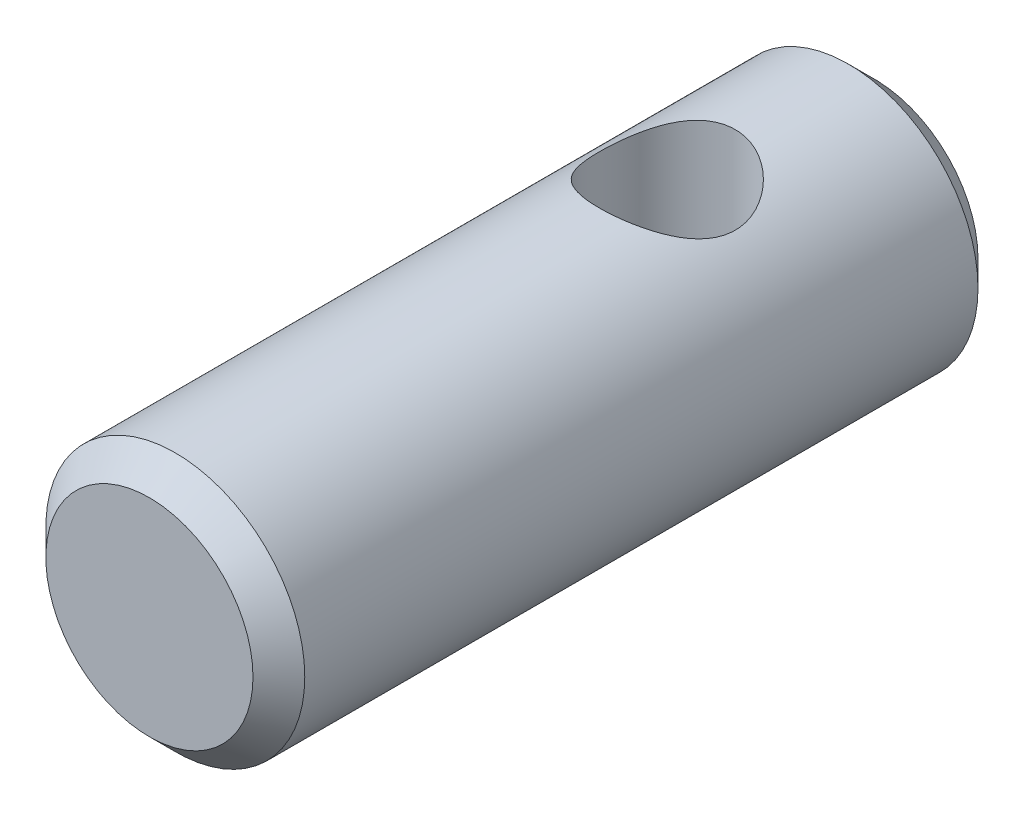
ISO-10303-21;
HEADER;
FILE_DESCRIPTION(('STEP AP214'),'2;1');
FILE_NAME('part.step','',(''),(''),'','','');
FILE_SCHEMA(('AUTOMOTIVE_DESIGN { 1 0 10303 214 1 1 1 1 }'));
ENDSEC;
DATA;
#1=APPLICATION_CONTEXT('core data for automotive mechanical design processes');
#2=APPLICATION_PROTOCOL_DEFINITION('international standard','automotive_design',2000,#1);
#3=PRODUCT_CONTEXT('',#1,'mechanical');
#4=PRODUCT('Part','Part','',(#3));
#5=PRODUCT_RELATED_PRODUCT_CATEGORY('part','',(#4));
#6=PRODUCT_DEFINITION_FORMATION('','',#4);
#7=PRODUCT_DEFINITION_CONTEXT('part definition',#1,'design');
#8=PRODUCT_DEFINITION('design','',#6,#7);
#9=PRODUCT_DEFINITION_SHAPE('','',#8);
#10=(LENGTH_UNIT() NAMED_UNIT(*) SI_UNIT(.MILLI.,.METRE.));
#11=(NAMED_UNIT(*) PLANE_ANGLE_UNIT() SI_UNIT($,.RADIAN.));
#12=(NAMED_UNIT(*) SI_UNIT($,.STERADIAN.) SOLID_ANGLE_UNIT());
#13=UNCERTAINTY_MEASURE_WITH_UNIT(LENGTH_MEASURE(1.E-05),#10,'distance_accuracy_value','');
#14=(GEOMETRIC_REPRESENTATION_CONTEXT(3) GLOBAL_UNCERTAINTY_ASSIGNED_CONTEXT((#13)) GLOBAL_UNIT_ASSIGNED_CONTEXT((#10,
#11,#12)) REPRESENTATION_CONTEXT('',''));
#15=CARTESIAN_POINT('',(0.,0.,0.));
#16=DIRECTION('',(0.,0.,1.));
#17=DIRECTION('',(1.,0.,0.));
#18=AXIS2_PLACEMENT_3D('',#15,#16,#17);
#19=CARTESIAN_POINT('',(0.,0.,56.));
#20=DIRECTION('',(0.,0.,-1.));
#21=DIRECTION('',(-1.,0.,0.));
#22=AXIS2_PLACEMENT_3D('',#19,#20,#21);
#23=CYLINDRICAL_SURFACE('',#22,10.);
#24=CARTESIAN_POINT('',(0.,0.,54.));
#25=DIRECTION('',(0.,0.,1.));
#26=DIRECTION('',(1.,0.,0.));
#27=AXIS2_PLACEMENT_3D('',#24,#25,#26);
#28=CIRCLE('',#27,10.);
#29=CARTESIAN_POINT('',(10.,0.,54.));
#30=VERTEX_POINT('',#29);
#31=EDGE_CURVE('E50',#30,#30,#28,.F.);
#32=ORIENTED_EDGE('',*,*,#31,.T.);
#33=EDGE_LOOP('',(#32));
#34=FACE_BOUND('',#33,.T.);
#35=CARTESIAN_POINT('',(0.,0.,1.99999999999999));
#36=DIRECTION('',(0.,0.,1.));
#37=DIRECTION('',(1.,0.,0.));
#38=AXIS2_PLACEMENT_3D('',#35,#36,#37);
#39=CIRCLE('',#38,10.);
#40=CARTESIAN_POINT('',(10.,0.,1.99999999999999));
#41=VERTEX_POINT('',#40);
#42=EDGE_CURVE('E51',#41,#41,#39,.T.);
#43=ORIENTED_EDGE('',*,*,#42,.T.);
#44=EDGE_LOOP('',(#43));
#45=FACE_BOUND('',#44,.T.);
#46=CARTESIAN_POINT('',(0.,-10.,21.25));
#47=CARTESIAN_POINT('',(0.137219280547153,-10.0000002272335,21.2500002845405));
#48=CARTESIAN_POINT('',(0.274435419117508,-9.9971695390607,21.244614606331));
#49=CARTESIAN_POINT('',(0.547846222323781,-9.98591963414679,21.2231383953593));
#50=CARTESIAN_POINT('',(0.684040493235206,-9.97749836499467,21.2070439311885));
#51=CARTESIAN_POINT('',(0.954484268200273,-9.95526954825004,21.1643222587016));
#52=CARTESIAN_POINT('',(1.08873124630636,-9.94145555844572,21.1376824522521));
#53=CARTESIAN_POINT('',(1.35420731073398,-9.90878502481806,21.0741759100838));
#54=CARTESIAN_POINT('',(1.48543513996533,-9.88992642039346,21.037304994978));
#55=CARTESIAN_POINT('',(1.74338589936232,-9.84772073139797,20.953926916141));
#56=CARTESIAN_POINT('',(1.87012634391849,-9.82439408650479,20.9074635617848));
#57=CARTESIAN_POINT('',(2.11899910335566,-9.77374047241918,20.8052537810732));
#58=CARTESIAN_POINT('',(2.24112965821982,-9.74641199440784,20.7495038522873));
#59=CARTESIAN_POINT('',(2.59949324496559,-9.65934198911403,20.5690867282639));
#60=CARTESIAN_POINT('',(2.82796520762876,-9.59447028649094,20.4311649077595));
#61=CARTESIAN_POINT('',(3.27372275797712,-9.45204211778156,20.1139922398255));
#62=CARTESIAN_POINT('',(3.48932750449225,-9.37393643487358,19.9326443666005));
#63=CARTESIAN_POINT('',(3.8886458044364,-9.21545596865336,19.5383334829643));
#64=CARTESIAN_POINT('',(4.07233236069242,-9.13507933066736,19.3253439890081));
#65=CARTESIAN_POINT('',(4.41885642960393,-8.97292923888063,18.8512480626824));
#66=CARTESIAN_POINT('',(4.57845425792897,-8.89165111021945,18.5875602559427));
#67=CARTESIAN_POINT('',(4.78231536149079,-8.78267726364413,18.1716075663925));
#68=CARTESIAN_POINT('',(4.84436102124095,-8.74850075709137,18.0295030388187));
#69=CARTESIAN_POINT('',(4.95595024092318,-8.68577293511993,17.7393030342969));
#70=CARTESIAN_POINT('',(5.00550154057647,-8.65721813970725,17.5912113324525));
#71=CARTESIAN_POINT('',(5.08878465482483,-8.60851077322863,17.2993729510763));
#72=CARTESIAN_POINT('',(5.12330119908315,-8.58794984553599,17.1559180994452));
#73=CARTESIAN_POINT('',(5.18020997914699,-8.55374369431526,16.8658774929062));
#74=CARTESIAN_POINT('',(5.20260898139194,-8.54009461148355,16.7192935329284));
#75=CARTESIAN_POINT('',(5.23492209789572,-8.52032581020631,16.4243606895251));
#76=CARTESIAN_POINT('',(5.24484570818525,-8.51420036499284,16.2760132353741));
#77=CARTESIAN_POINT('',(5.25205946869656,-8.50975281069956,15.9789018663673));
#78=CARTESIAN_POINT('',(5.24935106056602,-8.51142981115412,15.8301380009715));
#79=CARTESIAN_POINT('',(5.23257907023163,-8.5217479943958,15.5537912805343));
#80=CARTESIAN_POINT('',(5.22010486854874,-8.52941410986321,15.426071367475));
#81=CARTESIAN_POINT('',(5.18592245284569,-8.55024031855141,15.1722883834829));
#82=CARTESIAN_POINT('',(5.16421138189128,-8.56340211154436,15.0462258376151));
#83=CARTESIAN_POINT('',(5.11181617148469,-8.59478129237691,14.7966330629832));
#84=CARTESIAN_POINT('',(5.08113266753343,-8.61299832215873,14.6731026555353));
#85=CARTESIAN_POINT('',(5.01112590957965,-8.65391561205324,14.4292574721334));
#86=CARTESIAN_POINT('',(4.97179923690138,-8.67661764578174,14.3089439897666));
#87=CARTESIAN_POINT('',(4.83944266050791,-8.75158613496986,13.9484926319502));
#88=CARTESIAN_POINT('',(4.7331971950735,-8.80998221055456,13.7143322078009));
#89=CARTESIAN_POINT('',(4.48927913110239,-8.93673383412094,13.2661129763646));
#90=CARTESIAN_POINT('',(4.35159249631468,-9.00509382533885,13.0520632074793));
#91=CARTESIAN_POINT('',(4.02599923880666,-9.15575739072048,12.6180678022914));
#92=CARTESIAN_POINT('',(3.83374090515359,-9.23866411313319,12.4015852559708));
#93=CARTESIAN_POINT('',(3.41536670121867,-9.40135838816874,12.0023342528049));
#94=CARTESIAN_POINT('',(3.18923148995555,-9.48114412592955,11.8195851889832));
#95=CARTESIAN_POINT('',(2.821282740588,-9.59469562525509,11.5698133976322));
#96=CARTESIAN_POINT('',(2.68996216013096,-9.63242744398394,11.4888434006179));
#97=CARTESIAN_POINT('',(2.41986332749828,-9.70379978677848,11.3383880146168));
#98=CARTESIAN_POINT('',(2.28108827753964,-9.73744204764833,11.2688977457436));
#99=CARTESIAN_POINT('',(1.99703485726557,-9.79964224031448,11.1421678788624));
#100=CARTESIAN_POINT('',(1.85175947518982,-9.82820247889612,11.0849227202681));
#101=CARTESIAN_POINT('',(1.55574231468487,-9.87938315597843,10.9833638548017));
#102=CARTESIAN_POINT('',(1.40500124075675,-9.90200435691644,10.939048487957));
#103=CARTESIAN_POINT('',(1.11282934307188,-9.93888050639706,10.8672906984546));
#104=CARTESIAN_POINT('',(0.971749460230005,-9.95369724432438,10.8387051082509));
#105=CARTESIAN_POINT('',(0.687234152071724,-9.97737832564566,10.7931815930195));
#106=CARTESIAN_POINT('',(0.543798965935319,-9.98624326965873,10.7762424926943));
#107=CARTESIAN_POINT('',(0.255835151509784,-9.9977649691323,10.7542501032815));
#108=CARTESIAN_POINT('',(0.111307032752615,-10.0004244577754,10.7491915814063));
#109=CARTESIAN_POINT('',(-0.177649036404393,-9.99946551039621,10.7510180045486));
#110=CARTESIAN_POINT('',(-0.322076991762344,-9.99584741118279,10.7579023088026));
#111=CARTESIAN_POINT('',(-0.596977627902548,-9.98302883233932,10.7823894009097));
#112=CARTESIAN_POINT('',(-0.727564346720147,-9.97434520954031,10.7990002755381));
#113=CARTESIAN_POINT('',(-0.986752417901722,-9.95204728968371,10.8418917496917));
#114=CARTESIAN_POINT('',(-1.11535313429704,-9.93843144599325,10.8681753824162));
#115=CARTESIAN_POINT('',(-1.36965004237689,-9.90658705292847,10.9301208766084));
#116=CARTESIAN_POINT('',(-1.4953471268205,-9.88835994251531,10.9657798126174));
#117=CARTESIAN_POINT('',(-1.74314372577149,-9.84770291270563,11.0461184149203));
#118=CARTESIAN_POINT('',(-1.86524183923142,-9.82527138093231,11.0908015424625));
#119=CARTESIAN_POINT('',(-2.23123711650007,-9.75112230193064,11.240316825719));
#120=CARTESIAN_POINT('',(-2.46841439744369,-9.69338463506806,11.3590433850495));
#121=CARTESIAN_POINT('',(-2.92006961741366,-9.56704734835907,11.6290622439496));
#122=CARTESIAN_POINT('',(-3.13453840111886,-9.49844337518584,11.7803676042087));
#123=CARTESIAN_POINT('',(-3.55886678955075,-9.34827580923661,12.1295715799768));
#124=CARTESIAN_POINT('',(-3.76585720791017,-9.26610842953409,12.3307004883061));
#125=CARTESIAN_POINT('',(-4.14465083180736,-9.10299232838763,12.7646733438667));
#126=CARTESIAN_POINT('',(-4.31642352057216,-9.02204471969024,12.9975445078946));
#127=CARTESIAN_POINT('',(-4.54921678298438,-8.90577435633367,13.3749564890276));
#128=CARTESIAN_POINT('',(-4.6244388087147,-8.86683357688885,13.5098103007094));
#129=CARTESIAN_POINT('',(-4.76308083496289,-8.7931345699769,13.7865235798825));
#130=CARTESIAN_POINT('',(-4.82650617229413,-8.75837445370803,13.9283798425349));
#131=CARTESIAN_POINT('',(-4.94081379482617,-8.69440356931228,14.2181203619124));
#132=CARTESIAN_POINT('',(-4.99170730203359,-8.66518784171106,14.3659990863072));
#133=CARTESIAN_POINT('',(-5.08032094735002,-8.61353453429228,14.6668057821361));
#134=CARTESIAN_POINT('',(-5.11804336108919,-8.59109578367589,14.8197328763379));
#135=CARTESIAN_POINT('',(-5.17667803179201,-8.55587841408529,15.114123629598));
#136=CARTESIAN_POINT('',(-5.19887396728424,-8.54236940354325,15.2552448007445));
#137=CARTESIAN_POINT('',(-5.23170136755015,-8.52230458141236,15.5393099760195));
#138=CARTESIAN_POINT('',(-5.24233433352715,-8.51574786721987,15.6822537410848));
#139=CARTESIAN_POINT('',(-5.25185951233148,-8.50987680634923,15.9686108559526));
#140=CARTESIAN_POINT('',(-5.25075745481041,-8.51055892529399,16.1120239424167));
#141=CARTESIAN_POINT('',(-5.23684562254051,-8.51912638319485,16.398056141514));
#142=CARTESIAN_POINT('',(-5.22403653550511,-8.52701129903249,16.5406753002904));
#143=CARTESIAN_POINT('',(-5.18905861916022,-8.54833517431968,16.8075526419432));
#144=CARTESIAN_POINT('',(-5.16813575164992,-8.5610310262324,16.9320359741887));
#145=CARTESIAN_POINT('',(-5.11754218486671,-8.59136907943889,17.1786107034704));
#146=CARTESIAN_POINT('',(-5.0878688274224,-8.60901278368161,17.3007013616383));
#147=CARTESIAN_POINT('',(-4.98617367311396,-8.66858187281142,17.6622746890925));
#148=CARTESIAN_POINT('',(-4.90145556802352,-8.71715897973571,17.8972171923239));
#149=CARTESIAN_POINT('',(-4.69456138578904,-8.83039079036659,18.3650285592195));
#150=CARTESIAN_POINT('',(-4.57029454343953,-8.89589043768955,18.5967527275334));
#151=CARTESIAN_POINT('',(-4.28992761428728,-9.03443201618363,19.0376472698748));
#152=CARTESIAN_POINT('',(-4.13381040597987,-9.10747799349605,19.2468054204548));
#153=CARTESIAN_POINT('',(-3.76892931535455,-9.26498416164771,19.6668056172768));
#154=CARTESIAN_POINT('',(-3.55586671949328,-9.34962231131358,19.8738577757245));
#155=CARTESIAN_POINT('',(-3.09590888201791,-9.51181668814184,20.2504194945182));
#156=CARTESIAN_POINT('',(-2.84899294804858,-9.58936853521662,20.4199059262879));
#157=CARTESIAN_POINT('',(-2.45489845847901,-9.69497778028643,20.6432164783478));
#158=CARTESIAN_POINT('',(-2.31807696854077,-9.72867771558496,20.7130413299976));
#159=CARTESIAN_POINT('',(-2.03793218201021,-9.79118868583265,20.8407633736319));
#160=CARTESIAN_POINT('',(-1.89461212988962,-9.82000212708188,20.8986664393929));
#161=CARTESIAN_POINT('',(-1.60279401104823,-9.8718274054918,21.001745186262));
#162=CARTESIAN_POINT('',(-1.45430732159531,-9.8948511724765,21.0469470615697));
#163=CARTESIAN_POINT('',(-1.15317060054867,-9.9344468208744,21.1241423051091));
#164=CARTESIAN_POINT('',(-1.00052299145191,-9.95102237408543,21.1561431909917));
#165=CARTESIAN_POINT('',(-0.706948892559235,-9.9759631073553,21.2041056127254));
#166=CARTESIAN_POINT('',(-0.566275097942629,-9.98495530017708,21.2212954311786));
#167=CARTESIAN_POINT('',(-0.283733098336377,-9.99697368746327,21.2442425896913));
#168=CARTESIAN_POINT('',(-0.141864870006832,-9.99999976507347,21.2499997058263));
#169=CARTESIAN_POINT('',(0.,-10.,21.25));
#170=B_SPLINE_CURVE_WITH_KNOTS('',3,(#46,#47,#48,#49,#50,#51,#52,#53,#54,#55,#56,#57,#58,#59,
#60,#61,#62,#63,#64,#65,#66,#67,#68,#69,#70,#71,#72,#73,#74,#75,#76,#77,#78,#79,#80,#81,#82,#83,
#84,#85,#86,#87,#88,#89,#90,#91,#92,#93,#94,#95,#96,#97,#98,#99,#100,#101,#102,#103,#104,#105,
#106,#107,#108,#109,#110,#111,#112,#113,#114,#115,#116,#117,#118,#119,#120,#121,#122,#123,#124,
#125,#126,#127,#128,#129,#130,#131,#132,#133,#134,#135,#136,#137,#138,#139,#140,#141,#142,#143,
#144,#145,#146,#147,#148,#149,#150,#151,#152,#153,#154,#155,#156,#157,#158,#159,#160,#161,#162,
#163,#164,#165,#166,#167,#168,#169),.UNSPECIFIED.,.T.,.F.,(4,2,2,2,2,2,2,2,2,2,2,2,2,2,2,2,2,2,
2,2,2,2,2,2,2,2,2,2,2,2,2,2,2,2,2,2,2,2,2,2,2,2,2,2,2,2,2,2,2,2,2,2,2,2,2,2,2,2,2,2,2,4),(0.,
0.411518545933161,0.823188251936375,1.23535125612146,1.6476828765493,2.05817143133696,
2.46881515382125,3.28925857265437,4.16279834004599,5.03707340942756,5.98799664373627,
6.46377153903549,6.93925098407663,7.38552525893882,7.83155007620077,8.2772351818966,
8.72286942436893,9.10808235596051,9.49341451940308,9.8787193970855,10.2641769514919,
11.0518764559294,11.8399283021686,12.7396564856037,13.6399003132389,14.1158328503485,
14.591562551084,15.067075758997,15.542527891946,15.9760601737939,16.4095486996027,
16.8428462600368,17.2761205736583,17.6714347685004,18.0668730323905,18.4621880503312,
18.8576549811517,19.6683496017933,20.4793698332679,21.3758847965833,22.2731733526402,
22.750383935953,23.2273781016115,23.7039435622231,24.1804266436458,24.6102867369871,
25.0400910155598,25.4696854508541,25.8992546518331,26.27941671829,26.6596943872714,
27.4197738215506,28.2296595066908,29.0399817071355,29.9626916334695,30.8859680881548,
31.3572036982906,31.8282065755557,32.298230832392,32.7679870507957,33.1934293164578,
33.6188799148826),.UNSPECIFIED.);
#171=CARTESIAN_POINT('',(0.,-10.,21.25));
#172=VERTEX_POINT('',#171);
#173=EDGE_CURVE('E58',#172,#172,#170,.T.);
#174=ORIENTED_EDGE('',*,*,#173,.T.);
#175=EDGE_LOOP('',(#174));
#176=FACE_BOUND('',#175,.T.);
#177=CARTESIAN_POINT('',(0.,10.,21.25));
#178=CARTESIAN_POINT('',(-0.137219280547153,10.0000002272335,21.2500002845405));
#179=CARTESIAN_POINT('',(-0.274435419117508,9.9971695390607,21.244614606331));
#180=CARTESIAN_POINT('',(-0.547846222323781,9.98591963414679,21.2231383953593));
#181=CARTESIAN_POINT('',(-0.684040493235206,9.97749836499467,21.2070439311885));
#182=CARTESIAN_POINT('',(-0.954484268200274,9.95526954825004,21.1643222587016));
#183=CARTESIAN_POINT('',(-1.08873124630636,9.94145555844572,21.1376824522521));
#184=CARTESIAN_POINT('',(-1.35420731073399,9.90878502481806,21.0741759100838));
#185=CARTESIAN_POINT('',(-1.48543513996533,9.88992642039346,21.037304994978));
#186=CARTESIAN_POINT('',(-1.74338589936232,9.84772073139797,20.953926916141));
#187=CARTESIAN_POINT('',(-1.87012634391849,9.82439408650479,20.9074635617848));
#188=CARTESIAN_POINT('',(-2.11899910335566,9.77374047241918,20.8052537810732));
#189=CARTESIAN_POINT('',(-2.24112965821982,9.74641199440784,20.7495038522873));
#190=CARTESIAN_POINT('',(-2.59949324496559,9.65934198911403,20.5690867282639));
#191=CARTESIAN_POINT('',(-2.82796520762876,9.59447028649094,20.4311649077595));
#192=CARTESIAN_POINT('',(-3.27372275797712,9.45204211778156,20.1139922398255));
#193=CARTESIAN_POINT('',(-3.48932750449225,9.37393643487358,19.9326443666005));
#194=CARTESIAN_POINT('',(-3.8886458044364,9.21545596865336,19.5383334829643));
#195=CARTESIAN_POINT('',(-4.07233236069242,9.13507933066736,19.3253439890081));
#196=CARTESIAN_POINT('',(-4.41885642960393,8.97292923888063,18.8512480626824));
#197=CARTESIAN_POINT('',(-4.57845425792897,8.89165111021945,18.5875602559427));
#198=CARTESIAN_POINT('',(-4.78231536149079,8.78267726364413,18.1716075663925));
#199=CARTESIAN_POINT('',(-4.84436102124095,8.74850075709137,18.0295030388187));
#200=CARTESIAN_POINT('',(-4.95595024092318,8.68577293511993,17.7393030342969));
#201=CARTESIAN_POINT('',(-5.00550154057647,8.65721813970725,17.5912113324525));
#202=CARTESIAN_POINT('',(-5.08878465482483,8.60851077322863,17.2993729510763));
#203=CARTESIAN_POINT('',(-5.12330119908315,8.58794984553599,17.1559180994452));
#204=CARTESIAN_POINT('',(-5.18020997914699,8.55374369431526,16.8658774929062));
#205=CARTESIAN_POINT('',(-5.20260898139194,8.54009461148355,16.7192935329284));
#206=CARTESIAN_POINT('',(-5.23492209789572,8.52032581020631,16.4243606895251));
#207=CARTESIAN_POINT('',(-5.24484570818525,8.51420036499284,16.2760132353741));
#208=CARTESIAN_POINT('',(-5.25205946869656,8.50975281069956,15.9789018663673));
#209=CARTESIAN_POINT('',(-5.24935106056602,8.51142981115412,15.8301380009715));
#210=CARTESIAN_POINT('',(-5.23257907023163,8.5217479943958,15.5537912805343));
#211=CARTESIAN_POINT('',(-5.22010486854874,8.52941410986321,15.426071367475));
#212=CARTESIAN_POINT('',(-5.18592245284569,8.55024031855141,15.1722883834829));
#213=CARTESIAN_POINT('',(-5.16421138189128,8.56340211154436,15.0462258376151));
#214=CARTESIAN_POINT('',(-5.11181617148469,8.59478129237691,14.7966330629832));
#215=CARTESIAN_POINT('',(-5.08113266753343,8.61299832215873,14.6731026555353));
#216=CARTESIAN_POINT('',(-5.01112590957965,8.65391561205324,14.4292574721334));
#217=CARTESIAN_POINT('',(-4.97179923690138,8.67661764578174,14.3089439897666));
#218=CARTESIAN_POINT('',(-4.83944266050791,8.75158613496986,13.9484926319502));
#219=CARTESIAN_POINT('',(-4.7331971950735,8.80998221055456,13.7143322078009));
#220=CARTESIAN_POINT('',(-4.48927913110239,8.93673383412094,13.2661129763646));
#221=CARTESIAN_POINT('',(-4.35159249631468,9.00509382533885,13.0520632074793));
#222=CARTESIAN_POINT('',(-4.02599923880666,9.15575739072048,12.6180678022914));
#223=CARTESIAN_POINT('',(-3.83374090515359,9.23866411313319,12.4015852559708));
#224=CARTESIAN_POINT('',(-3.41536670121867,9.40135838816874,12.0023342528049));
#225=CARTESIAN_POINT('',(-3.18923148995555,9.48114412592955,11.8195851889832));
#226=CARTESIAN_POINT('',(-2.821282740588,9.59469562525509,11.5698133976322));
#227=CARTESIAN_POINT('',(-2.68996216013096,9.63242744398394,11.4888434006179));
#228=CARTESIAN_POINT('',(-2.41986332749828,9.70379978677848,11.3383880146168));
#229=CARTESIAN_POINT('',(-2.28108827753964,9.73744204764833,11.2688977457436));
#230=CARTESIAN_POINT('',(-1.99703485726557,9.79964224031448,11.1421678788624));
#231=CARTESIAN_POINT('',(-1.85175947518982,9.82820247889612,11.0849227202681));
#232=CARTESIAN_POINT('',(-1.55574231468487,9.87938315597843,10.9833638548017));
#233=CARTESIAN_POINT('',(-1.40500124075675,9.90200435691644,10.939048487957));
#234=CARTESIAN_POINT('',(-1.11282934307188,9.93888050639706,10.8672906984546));
#235=CARTESIAN_POINT('',(-0.971749460230005,9.95369724432438,10.8387051082509));
#236=CARTESIAN_POINT('',(-0.687234152071724,9.97737832564566,10.7931815930195));
#237=CARTESIAN_POINT('',(-0.543798965935319,9.98624326965873,10.7762424926943));
#238=CARTESIAN_POINT('',(-0.255835151509784,9.9977649691323,10.7542501032815));
#239=CARTESIAN_POINT('',(-0.111307032752615,10.0004244577754,10.7491915814063));
#240=CARTESIAN_POINT('',(0.177649036404393,9.99946551039621,10.7510180045486));
#241=CARTESIAN_POINT('',(0.322076991762344,9.99584741118279,10.7579023088026));
#242=CARTESIAN_POINT('',(0.596977627902548,9.98302883233932,10.7823894009097));
#243=CARTESIAN_POINT('',(0.727564346720147,9.97434520954031,10.7990002755381));
#244=CARTESIAN_POINT('',(0.986752417901722,9.95204728968371,10.8418917496917));
#245=CARTESIAN_POINT('',(1.11535313429704,9.93843144599325,10.8681753824162));
#246=CARTESIAN_POINT('',(1.36965004237689,9.90658705292847,10.9301208766084));
#247=CARTESIAN_POINT('',(1.4953471268205,9.88835994251531,10.9657798126174));
#248=CARTESIAN_POINT('',(1.74314372577149,9.84770291270563,11.0461184149203));
#249=CARTESIAN_POINT('',(1.86524183923142,9.82527138093231,11.0908015424625));
#250=CARTESIAN_POINT('',(2.23123711650007,9.75112230193064,11.240316825719));
#251=CARTESIAN_POINT('',(2.46841439744369,9.69338463506806,11.3590433850495));
#252=CARTESIAN_POINT('',(2.92006961741366,9.56704734835907,11.6290622439496));
#253=CARTESIAN_POINT('',(3.13453840111886,9.49844337518584,11.7803676042087));
#254=CARTESIAN_POINT('',(3.55886678955075,9.34827580923661,12.1295715799768));
#255=CARTESIAN_POINT('',(3.76585720791017,9.26610842953409,12.3307004883061));
#256=CARTESIAN_POINT('',(4.14465083180736,9.10299232838763,12.7646733438667));
#257=CARTESIAN_POINT('',(4.31642352057216,9.02204471969024,12.9975445078946));
#258=CARTESIAN_POINT('',(4.54921678298438,8.90577435633367,13.3749564890276));
#259=CARTESIAN_POINT('',(4.6244388087147,8.86683357688885,13.5098103007094));
#260=CARTESIAN_POINT('',(4.76308083496289,8.7931345699769,13.7865235798825));
#261=CARTESIAN_POINT('',(4.82650617229413,8.75837445370803,13.9283798425349));
#262=CARTESIAN_POINT('',(4.94081379482617,8.69440356931228,14.2181203619124));
#263=CARTESIAN_POINT('',(4.99170730203359,8.66518784171106,14.3659990863072));
#264=CARTESIAN_POINT('',(5.08032094735002,8.61353453429228,14.6668057821361));
#265=CARTESIAN_POINT('',(5.11804336108919,8.59109578367589,14.8197328763379));
#266=CARTESIAN_POINT('',(5.17667803179201,8.55587841408529,15.114123629598));
#267=CARTESIAN_POINT('',(5.19887396728424,8.54236940354325,15.2552448007445));
#268=CARTESIAN_POINT('',(5.23170136755015,8.52230458141236,15.5393099760195));
#269=CARTESIAN_POINT('',(5.24233433352715,8.51574786721987,15.6822537410848));
#270=CARTESIAN_POINT('',(5.25185951233148,8.50987680634923,15.9686108559526));
#271=CARTESIAN_POINT('',(5.25075745481041,8.51055892529399,16.1120239424167));
#272=CARTESIAN_POINT('',(5.23684562254051,8.51912638319485,16.398056141514));
#273=CARTESIAN_POINT('',(5.22403653550511,8.52701129903249,16.5406753002904));
#274=CARTESIAN_POINT('',(5.18905861916022,8.54833517431968,16.8075526419432));
#275=CARTESIAN_POINT('',(5.16813575164992,8.5610310262324,16.9320359741887));
#276=CARTESIAN_POINT('',(5.11754218486671,8.59136907943889,17.1786107034704));
#277=CARTESIAN_POINT('',(5.0878688274224,8.60901278368161,17.3007013616383));
#278=CARTESIAN_POINT('',(4.98617367311396,8.66858187281142,17.6622746890925));
#279=CARTESIAN_POINT('',(4.90145556802352,8.71715897973571,17.8972171923239));
#280=CARTESIAN_POINT('',(4.69456138578904,8.83039079036659,18.3650285592195));
#281=CARTESIAN_POINT('',(4.57029454343953,8.89589043768955,18.5967527275334));
#282=CARTESIAN_POINT('',(4.28992761428728,9.03443201618363,19.0376472698748));
#283=CARTESIAN_POINT('',(4.13381040597987,9.10747799349605,19.2468054204548));
#284=CARTESIAN_POINT('',(3.76892931535455,9.26498416164771,19.6668056172768));
#285=CARTESIAN_POINT('',(3.55586671949328,9.34962231131358,19.8738577757245));
#286=CARTESIAN_POINT('',(3.09590888201791,9.51181668814184,20.2504194945182));
#287=CARTESIAN_POINT('',(2.84899294804858,9.58936853521662,20.4199059262879));
#288=CARTESIAN_POINT('',(2.45489845847901,9.69497778028643,20.6432164783478));
#289=CARTESIAN_POINT('',(2.31807696854077,9.72867771558496,20.7130413299976));
#290=CARTESIAN_POINT('',(2.03793218201021,9.79118868583265,20.8407633736319));
#291=CARTESIAN_POINT('',(1.89461212988962,9.82000212708188,20.8986664393929));
#292=CARTESIAN_POINT('',(1.60279401104823,9.8718274054918,21.001745186262));
#293=CARTESIAN_POINT('',(1.45430732159531,9.8948511724765,21.0469470615697));
#294=CARTESIAN_POINT('',(1.15317060054867,9.9344468208744,21.1241423051091));
#295=CARTESIAN_POINT('',(1.00052299145191,9.95102237408543,21.1561431909917));
#296=CARTESIAN_POINT('',(0.706948892559235,9.9759631073553,21.2041056127254));
#297=CARTESIAN_POINT('',(0.566275097942629,9.98495530017709,21.2212954311786));
#298=CARTESIAN_POINT('',(0.283733098336377,9.99697368746327,21.2442425896913));
#299=CARTESIAN_POINT('',(0.141864870006832,9.99999976507347,21.2499997058263));
#300=CARTESIAN_POINT('',(0.,10.,21.25));
#301=B_SPLINE_CURVE_WITH_KNOTS('',3,(#177,#178,#179,#180,#181,#182,#183,#184,#185,#186,#187,
#188,#189,#190,#191,#192,#193,#194,#195,#196,#197,#198,#199,#200,#201,#202,#203,#204,#205,#206,
#207,#208,#209,#210,#211,#212,#213,#214,#215,#216,#217,#218,#219,#220,#221,#222,#223,#224,#225,
#226,#227,#228,#229,#230,#231,#232,#233,#234,#235,#236,#237,#238,#239,#240,#241,#242,#243,#244,
#245,#246,#247,#248,#249,#250,#251,#252,#253,#254,#255,#256,#257,#258,#259,#260,#261,#262,#263,
#264,#265,#266,#267,#268,#269,#270,#271,#272,#273,#274,#275,#276,#277,#278,#279,#280,#281,#282,
#283,#284,#285,#286,#287,#288,#289,#290,#291,#292,#293,#294,#295,#296,#297,#298,#299,#300),
.UNSPECIFIED.,.T.,.F.,(4,2,2,2,2,2,2,2,2,2,2,2,2,2,2,2,2,2,2,2,2,2,2,2,2,2,2,2,2,2,2,2,2,2,2,2,
2,2,2,2,2,2,2,2,2,2,2,2,2,2,2,2,2,2,2,2,2,2,2,2,2,4),(0.,0.411518545933161,0.823188251936375,
1.23535125612147,1.6476828765493,2.05817143133696,2.46881515382125,3.28925857265437,
4.16279834004599,5.03707340942756,5.98799664373627,6.46377153903549,6.93925098407663,
7.38552525893882,7.83155007620077,8.2772351818966,8.72286942436893,9.10808235596051,
9.49341451940308,9.8787193970855,10.2641769514919,11.0518764559294,11.8399283021686,
12.7396564856037,13.6399003132389,14.1158328503485,14.591562551084,15.067075758997,
15.542527891946,15.9760601737939,16.4095486996027,16.8428462600368,17.2761205736583,
17.6714347685004,18.0668730323905,18.4621880503312,18.8576549811517,19.6683496017933,
20.4793698332679,21.3758847965833,22.2731733526402,22.750383935953,23.2273781016115,
23.7039435622231,24.1804266436458,24.6102867369871,25.0400910155598,25.4696854508541,
25.8992546518331,26.27941671829,26.6596943872714,27.4197738215506,28.2296595066908,
29.0399817071355,29.9626916334695,30.8859680881548,31.3572036982906,31.8282065755557,
32.298230832392,32.7679870507957,33.1934293164578,33.6188799148826),.UNSPECIFIED.);
#302=CARTESIAN_POINT('',(0.,10.,21.25));
#303=VERTEX_POINT('',#302);
#304=EDGE_CURVE('E70',#303,#303,#301,.T.);
#305=ORIENTED_EDGE('',*,*,#304,.T.);
#306=EDGE_LOOP('',(#305));
#307=FACE_BOUND('',#306,.T.);
#308=ADVANCED_FACE('F39',(#34,#45,#176,#307),#23,.T.);
#309=CARTESIAN_POINT('',(0.,0.,56.));
#310=DIRECTION('',(0.,0.,1.));
#311=DIRECTION('',(1.,0.,0.));
#312=AXIS2_PLACEMENT_3D('',#309,#310,#311);
#313=PLANE('',#312);
#314=CARTESIAN_POINT('',(0.,0.,56.));
#315=DIRECTION('',(0.,0.,1.));
#316=DIRECTION('',(1.,0.,0.));
#317=AXIS2_PLACEMENT_3D('',#314,#315,#316);
#318=CIRCLE('',#317,7.99999999999999);
#319=CARTESIAN_POINT('',(7.99999999999999,0.,56.));
#320=VERTEX_POINT('',#319);
#321=EDGE_CURVE('E54',#320,#320,#318,.T.);
#322=ORIENTED_EDGE('',*,*,#321,.T.);
#323=EDGE_LOOP('',(#322));
#324=FACE_BOUND('',#323,.T.);
#325=ADVANCED_FACE('F84',(#324),#313,.T.);
#326=CARTESIAN_POINT('',(0.,0.,0.));
#327=DIRECTION('',(0.,0.,1.));
#328=DIRECTION('',(1.,0.,0.));
#329=AXIS2_PLACEMENT_3D('',#326,#327,#328);
#330=PLANE('',#329);
#331=CARTESIAN_POINT('',(0.,0.,0.));
#332=DIRECTION('',(0.,0.,1.));
#333=DIRECTION('',(1.,0.,0.));
#334=AXIS2_PLACEMENT_3D('',#331,#332,#333);
#335=CIRCLE('',#334,8.);
#336=CARTESIAN_POINT('',(8.,0.,0.));
#337=VERTEX_POINT('',#336);
#338=EDGE_CURVE('E10',#337,#337,#335,.F.);
#339=ORIENTED_EDGE('',*,*,#338,.T.);
#340=EDGE_LOOP('',(#339));
#341=FACE_BOUND('',#340,.T.);
#342=ADVANCED_FACE('F80',(#341),#330,.F.);
#343=CARTESIAN_POINT('',(0.,-10.,16.));
#344=DIRECTION('',(0.,1.,0.));
#345=DIRECTION('',(0.,0.,1.));
#346=AXIS2_PLACEMENT_3D('',#343,#344,#345);
#347=CYLINDRICAL_SURFACE('',#346,5.25);
#348=ORIENTED_EDGE('',*,*,#304,.F.);
#349=EDGE_LOOP('',(#348));
#350=FACE_BOUND('',#349,.T.);
#351=ORIENTED_EDGE('',*,*,#173,.F.);
#352=EDGE_LOOP('',(#351));
#353=FACE_BOUND('',#352,.T.);
#354=ADVANCED_FACE('F74',(#350,#353),#347,.F.);
#355=CARTESIAN_POINT('',(0.,0.,56.));
#356=DIRECTION('',(0.,0.,-1.));
#357=DIRECTION('',(-1.,0.,0.));
#358=AXIS2_PLACEMENT_3D('',#355,#356,#357);
#359=CONICAL_SURFACE('',#358,7.99999999999999,0.785398163397447);
#360=ORIENTED_EDGE('',*,*,#31,.F.);
#361=EDGE_LOOP('',(#360));
#362=FACE_BOUND('',#361,.T.);
#363=ORIENTED_EDGE('',*,*,#321,.F.);
#364=EDGE_LOOP('',(#363));
#365=FACE_BOUND('',#364,.T.);
#366=ADVANCED_FACE('F77',(#362,#365),#359,.T.);
#367=CARTESIAN_POINT('',(0.,0.,1.99999999999999));
#368=DIRECTION('',(0.,0.,1.));
#369=DIRECTION('',(1.,0.,0.));
#370=AXIS2_PLACEMENT_3D('',#367,#368,#369);
#371=CONICAL_SURFACE('',#370,10.,0.785398163397449);
#372=ORIENTED_EDGE('',*,*,#338,.F.);
#373=EDGE_LOOP('',(#372));
#374=FACE_BOUND('',#373,.T.);
#375=ORIENTED_EDGE('',*,*,#42,.F.);
#376=EDGE_LOOP('',(#375));
#377=FACE_BOUND('',#376,.T.);
#378=ADVANCED_FACE('F45',(#374,#377),#371,.T.);
#379=CLOSED_SHELL('',(#308,#325,#342,#354,#366,#378));
#380=MANIFOLD_SOLID_BREP('B2',#379);
#381=ADVANCED_BREP_SHAPE_REPRESENTATION('',(#18,#380),#14);
#382=SHAPE_DEFINITION_REPRESENTATION(#9,#381);
ENDSEC;
END-ISO-10303-21;
